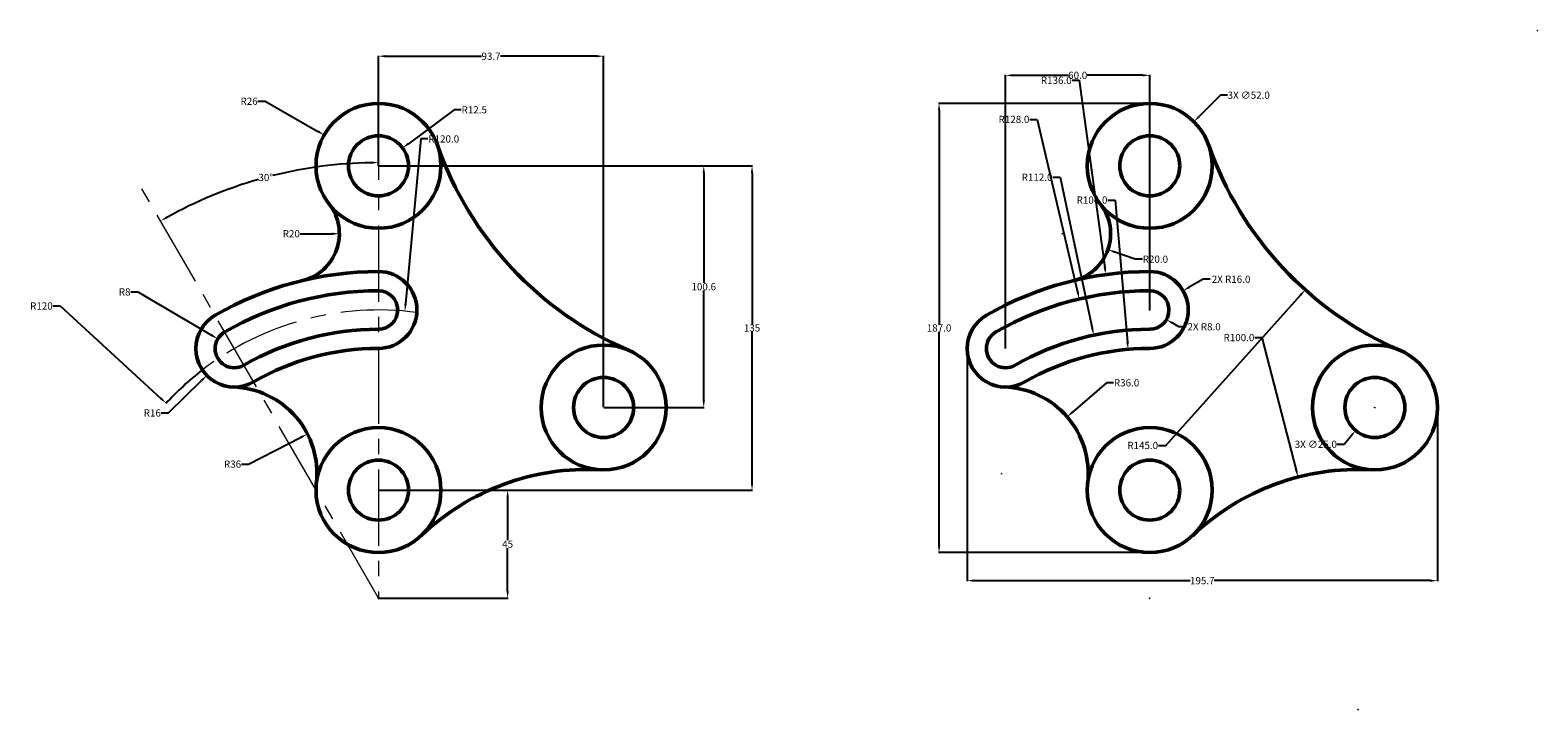
# Model space of a CAD drawing. Units: millimetres. Extents: x -10 to 618, y 0 to 283.
import ezdxf

# ---------------------------------------------------------------- set-up
doc = ezdxf.new("R2010")
doc.units = ezdxf.units.MM
doc.header["$MEASUREMENT"] = 0
doc.linetypes.add('CENTER', pattern=[50.8, 31.75, -6.35, 6.35, -6.35])
for name, color, linetype, lineweight in [('M-CNTR', 7, 'CENTER', 18), ('M-DIMS', 3, 'Continuous', 25), ('M-OUTL', 7, 'Continuous', 50)]:
    doc.layers.add(name, color=color, linetype=linetype, lineweight=lineweight)
doc.styles.get("Standard").update_dxf_attribs({"font": 'arial.ttf'})
doc.dimstyles.get("Standard").update_dxf_attribs({"dimtxt": 3, "dimasz": 3, "dimexe": 0.18, "dimexo": 0.0625, "dimgap": 0.09, "dimtad": 0, "dimtih": 1, "dimtoh": 1, "dimdec": 1, "dimdsep": 46, "dimtxsty": 'Standard', "dimcen": 0.09, "dimadec": 0, "dimazin": 0, "dimtfac": 1, "dimtdec": 1, "dimtofl": 0, "dimtmove": 0, "dimatfit": 3, "dimfxl": 1, "dimtolj": 1, "dimtzin": 0, "dimarcsym": 0})

# ---------------------------------------------------------------- blocks, each defined once
blk = doc.blocks.new('*D1')
at = {"layer": 'Defpoints', "color": 0, "transparency": 16777216}
for p in [(135.32, 252.15), (103.83, 224.75), (35.32, 219.36), (135.32, 46.15), (135.32, 46.15)]:
    blk.add_point(p, dxfattribs=at)
at = {"layer": 'M-DIMS', "color": 0, "lineweight": -2, "transparency": 16777216}
for start, end in [(90.94784, 104.01062), (105.99398, 119.05216)]:
    blk.add_arc((135.32, 46.15), 181.35, start, end, dxfattribs=at)
at = {"layer": 'M-DIMS', "color": 0, "transparency": 16777216}
for points in [[(132.32, 227.98), (132.33, 226.98), (135.32, 227.5)], [(47.51, 204.25), (47.01, 205.12), (44.65, 203.21)]]:
    blk.add_solid(points, dxfattribs=at)
at = {"layer": 'M-DIMS', "color": 0, "transparency": 16777216, "insert": (88.39, 221.32), "char_height": 3, "attachment_point": 5}
blk.add_mtext('\\A1;30°', dxfattribs=at)
blk = doc.blocks.new('*D2')
at = {"layer": 'Defpoints', "color": 0, "transparency": 16777216}
for p in [(99.04, 197.88), (119.04, 197.88)]:
    blk.add_point(p, dxfattribs=at)
at = {"layer": 'M-DIMS', "color": 0, "lineweight": -2, "transparency": 16777216}
blk.add_line((102.71, 197.88), (116.04, 197.88), dxfattribs=at)
at = {"layer": 'M-DIMS', "color": 0, "transparency": 16777216}
blk.add_solid([(116.04, 198.38), (116.04, 197.38), (119.04, 197.88)], dxfattribs=at)
at = {"layer": 'M-DIMS', "color": 0, "transparency": 16777216, "insert": (99.04, 197.88), "char_height": 3, "attachment_point": 5}
blk.add_mtext('\\A1;R20', dxfattribs=at)
blk = doc.blocks.new('*D3')
at = {"layer": 'Defpoints', "color": 0, "transparency": 16777216}
for p in [(135.32, 91.15), (189.08, 91.15), (135.32, 46.15)]:
    blk.add_point(p, dxfattribs=at)
at = {"layer": 'M-DIMS', "color": 0, "lineweight": -2, "transparency": 16777216}
for p, q in [((135.39, 91.15), (189.26, 91.15)), ((189.08, 88.15), (189.08, 70.27)), ((189.08, 49.15), (189.08, 67.04)), ((135.39, 46.15), (189.26, 46.15))]:
    blk.add_line(p, q, dxfattribs=at)
at = {"layer": 'M-DIMS', "color": 0, "transparency": 16777216}
for points in [[(188.58, 88.15), (189.58, 88.15), (189.08, 91.15)], [(188.58, 49.15), (189.58, 49.15), (189.08, 46.15)]]:
    blk.add_solid(points, dxfattribs=at)
at = {"layer": 'M-DIMS', "color": 0, "transparency": 16777216, "insert": (189.08, 68.65), "char_height": 3, "attachment_point": 5}
blk.add_mtext('\\A1;45', dxfattribs=at)
blk = doc.blocks.new('*D4')
at = {"layer": 'Defpoints', "color": 0, "transparency": 16777216}
for p in [(135.32, 226.15), (290.79, 226.15), (135.32, 91.15)]:
    blk.add_point(p, dxfattribs=at)
at = {"layer": 'M-DIMS', "color": 0, "lineweight": -2, "transparency": 16777216}
for p, q in [((135.39, 226.15), (290.97, 226.15)), ((290.79, 223.15), (290.79, 160.28)), ((290.79, 94.15), (290.79, 157.03)), ((135.39, 91.15), (290.97, 91.15))]:
    blk.add_line(p, q, dxfattribs=at)
at = {"layer": 'M-DIMS', "color": 0, "transparency": 16777216}
for points in [[(290.29, 223.15), (291.29, 223.15), (290.79, 226.15)], [(290.29, 94.15), (291.29, 94.15), (290.79, 91.15)]]:
    blk.add_solid(points, dxfattribs=at)
at = {"layer": 'M-DIMS', "color": 0, "transparency": 16777216, "insert": (290.79, 158.65), "char_height": 3, "attachment_point": 5}
blk.add_mtext('\\A1;135', dxfattribs=at)
blk = doc.blocks.new('*D5')
at = {"layer": 'Defpoints', "color": 0, "transparency": 16777216}
for p in [(135.32, 271.81), (135.32, 226.15), (229.02, 125.55)]:
    blk.add_point(p, dxfattribs=at)
at = {"layer": 'M-DIMS', "color": 0, "lineweight": -2, "transparency": 16777216}
for p, q in [((135.32, 226.22), (135.32, 271.99)), ((138.32, 271.81), (178.19, 271.81)), ((226.02, 271.81), (186.16, 271.81)), ((229.02, 125.62), (229.02, 271.99))]:
    blk.add_line(p, q, dxfattribs=at)
at = {"layer": 'M-DIMS', "color": 0, "transparency": 16777216}
for points in [[(138.32, 272.31), (138.32, 271.31), (135.32, 271.81)], [(226.02, 272.31), (226.02, 271.31), (229.02, 271.81)]]:
    blk.add_solid(points, dxfattribs=at)
at = {"layer": 'M-DIMS', "color": 0, "transparency": 16777216, "insert": (182.17, 271.81), "char_height": 3, "attachment_point": 5}
blk.add_mtext('\\A1;93.7', dxfattribs=at)
blk = doc.blocks.new('*D6')
at = {"layer": 'Defpoints', "color": 0, "transparency": 16777216}
for p in [(135.32, 226.15), (270.7, 226.15), (229.02, 125.55)]:
    blk.add_point(p, dxfattribs=at)
at = {"layer": 'M-DIMS', "color": 0, "lineweight": -2, "transparency": 16777216}
for p, q in [((135.39, 226.15), (270.88, 226.15)), ((270.7, 223.15), (270.7, 177.47)), ((270.7, 128.55), (270.7, 174.23)), ((229.09, 125.55), (270.88, 125.55))]:
    blk.add_line(p, q, dxfattribs=at)
at = {"layer": 'M-DIMS', "color": 0, "transparency": 16777216}
for points in [[(270.2, 223.15), (271.2, 223.15), (270.7, 226.15)], [(270.2, 128.55), (271.2, 128.55), (270.7, 125.55)]]:
    blk.add_solid(points, dxfattribs=at)
at = {"layer": 'M-DIMS', "color": 0, "transparency": 16777216, "insert": (270.7, 175.85), "char_height": 3, "attachment_point": 5}
blk.add_mtext('\\A1;100.6', dxfattribs=at)
blk = doc.blocks.new('*D7')
at = {"layer": 'Defpoints', "color": 0, "transparency": 16777216}
for p in [(75.32, 150.08), (63.87, 138.9)]:
    blk.add_point(p, dxfattribs=at)
at = {"layer": 'M-DIMS', "color": 0, "lineweight": -2, "transparency": 16777216}
for p, q in [((75.23, 150.08), (75.41, 150.08)), ((75.32, 149.99), (75.32, 150.17)), ((47.87, 123.28), (61.73, 136.8)), ((44.87, 123.28), (47.87, 123.28))]:
    blk.add_line(p, q, dxfattribs=at)
at = {"layer": 'M-DIMS', "color": 0, "transparency": 16777216}
blk.add_solid([(61.38, 137.16), (62.08, 136.45), (63.87, 138.9)], dxfattribs=at)
at = {"layer": 'M-DIMS', "color": 0, "transparency": 16777216, "insert": (41.2, 123.28), "char_height": 3, "attachment_point": 5}
blk.add_mtext('\\A1;R16', dxfattribs=at)
blk = doc.blocks.new('*D8')
at = {"layer": 'Defpoints', "color": 0, "transparency": 16777216}
for p in [(105.75, 114.53), (73.71, 98.1)]:
    blk.add_point(p, dxfattribs=at)
at = {"layer": 'M-DIMS', "color": 0, "lineweight": -2, "transparency": 16777216}
for p, q in [((81.25, 101.97), (103.08, 113.16)), ((78.25, 101.97), (81.25, 101.97))]:
    blk.add_line(p, q, dxfattribs=at)
at = {"layer": 'M-DIMS', "color": 0, "transparency": 16777216}
blk.add_solid([(102.85, 113.61), (103.31, 112.72), (105.75, 114.53)], dxfattribs=at)
at = {"layer": 'M-DIMS', "color": 0, "transparency": 16777216, "insert": (74.58, 101.97), "char_height": 3, "attachment_point": 5}
blk.add_mtext('\\A1;R36', dxfattribs=at)
blk = doc.blocks.new('*D9')
at = {"layer": 'Defpoints', "color": 0, "transparency": 16777216}
for p in [(46.95, 127.33), (135.32, 46.15)]:
    blk.add_point(p, dxfattribs=at)
at = {"layer": 'M-DIMS', "color": 0, "lineweight": -2, "transparency": 16777216}
for p, q in [((-0.11, 167.81), (2.89, 167.81)), ((2.89, 167.81), (44.74, 129.36)), ((135.23, 46.15), (135.41, 46.15)), ((135.32, 46.06), (135.32, 46.24))]:
    blk.add_line(p, q, dxfattribs=at)
blk.add_arc((135.32, 46.15), 120, 127.67495, 137.51567, dxfattribs=at)
at = {"layer": 'M-DIMS', "color": 0, "transparency": 16777216}
blk.add_solid([(45.08, 129.73), (44.4, 128.99), (46.95, 127.33)], dxfattribs=at)
at = {"layer": 'M-DIMS', "color": 0, "transparency": 16777216, "insert": (-4.95, 167.81), "char_height": 3, "attachment_point": 5}
blk.add_mtext('\\A1;R120', dxfattribs=at)
blk = doc.blocks.new('*D10')
at = {"layer": 'Defpoints', "color": 0, "transparency": 16777216}
for p in [(68.43, 154.13), (75.32, 150.08)]:
    blk.add_point(p, dxfattribs=at)
at = {"layer": 'M-DIMS', "color": 0, "lineweight": -2, "transparency": 16777216}
for p, q in [((32.2, 173.67), (35.2, 173.67)), ((35.2, 173.67), (65.84, 155.65)), ((75.23, 150.08), (75.41, 150.08)), ((75.32, 149.99), (75.32, 150.17))]:
    blk.add_line(p, q, dxfattribs=at)
at = {"layer": 'M-DIMS', "color": 0, "transparency": 16777216}
blk.add_solid([(66.1, 156.08), (65.59, 155.22), (68.43, 154.13)], dxfattribs=at)
at = {"layer": 'M-DIMS', "color": 0, "transparency": 16777216, "insert": (29.69, 173.67), "char_height": 3, "attachment_point": 5}
blk.add_mtext('\\A1;R8', dxfattribs=at)
blk = doc.blocks.new('*D11')
at = {"layer": 'Defpoints', "color": 0, "transparency": 16777216}
for p in [(112.74, 239.03), (135.32, 226.15)]:
    blk.add_point(p, dxfattribs=at)
at = {"layer": 'M-DIMS', "color": 0, "lineweight": -2, "transparency": 16777216}
for p, q in [((85.14, 253.05), (88.14, 253.05)), ((88.14, 253.05), (110.13, 240.52)), ((135.23, 226.15), (135.41, 226.15)), ((135.32, 226.06), (135.32, 226.24))]:
    blk.add_line(p, q, dxfattribs=at)
at = {"layer": 'M-DIMS', "color": 0, "transparency": 16777216}
blk.add_solid([(110.38, 240.95), (109.88, 240.08), (112.74, 239.03)], dxfattribs=at)
at = {"layer": 'M-DIMS', "color": 0, "transparency": 16777216, "insert": (81.47, 253.05), "char_height": 3, "attachment_point": 5}
blk.add_mtext('\\A1;R26', dxfattribs=at)
blk = doc.blocks.new('*D12')
at = {"layer": 'Defpoints', "color": 0, "transparency": 16777216}
for p in [(145.36, 233.6), (135.32, 226.15)]:
    blk.add_point(p, dxfattribs=at)
at = {"layer": 'M-DIMS', "color": 0, "lineweight": -2, "transparency": 16777216}
for p, q in [((166.76, 249.49), (147.77, 235.39)), ((169.76, 249.49), (166.76, 249.49)), ((135.23, 226.15), (135.41, 226.15)), ((135.32, 226.06), (135.32, 226.24))]:
    blk.add_line(p, q, dxfattribs=at)
at = {"layer": 'M-DIMS', "color": 0, "transparency": 16777216}
blk.add_solid([(147.47, 235.79), (148.07, 234.99), (145.36, 233.6)], dxfattribs=at)
at = {"layer": 'M-DIMS', "color": 0, "transparency": 16777216, "insert": (175.19, 249.49), "char_height": 3, "attachment_point": 5}
blk.add_mtext('\\A1;R12.5', dxfattribs=at)
blk = doc.blocks.new('LINKAGE-BRACKET-ARC-SLOT')
for centre, radius in [((76, 161), 26), ((76, 161), 12.5), ((169.7, 60.4), 26), ((169.7, 60.4), 12.5), ((76, 26), 26), ((76, 26), 12.5)]:
    blk.add_circle(centre, radius)
for centre, radius, start, end in [((237.43, 217.42), 145, 199.26409, 246.66823), ((39.72, 132.72), 20, 283.44875, 37.93262), ((76, -19), 136, 90, 120), ((76, 101), 16, 270, 90), ((76, -19), 128, 90, 120), ((76, 101), 8, 270, 90), ((16, 84.92), 16, 120, 300), ((16, 84.92), 8, 120, 300), ((76, -19), 112, 90, 120), ((76, -19), 104, 90, 120), ((14.39, 32.95), 36, 353.5657, 88.22634), ((162.72, -65.41), 100, 86.82559, 133.49373)]:
    blk.add_arc(centre, radius, start, end)
blk = doc.blocks.new('*D14')
at = {"layer": 'Defpoints', "color": 0, "transparency": 16777216}
for p in [(380.33, 150.08), (576.03, 125.55), (576.03, 53.45)]:
    blk.add_point(p, dxfattribs=at)
at = {"layer": 'M-DIMS', "color": 0, "lineweight": -2, "transparency": 16777216}
for p, q in [((380.33, 150.01), (380.33, 53.27)), ((576.03, 125.49), (576.03, 53.27)), ((383.33, 53.45), (473.17, 53.45)), ((573.03, 53.45), (483.19, 53.45))]:
    blk.add_line(p, q, dxfattribs=at)
at = {"layer": 'M-DIMS', "color": 0, "transparency": 16777216}
for points in [[(383.33, 53.95), (383.33, 52.95), (380.33, 53.45)], [(573.03, 53.95), (573.03, 52.95), (576.03, 53.45)]]:
    blk.add_solid(points, dxfattribs=at)
at = {"layer": 'M-DIMS', "color": 0, "transparency": 16777216, "insert": (478.18, 53.45), "char_height": 3, "attachment_point": 5}
blk.add_mtext('\\A1;195.7', dxfattribs=at)
blk = doc.blocks.new('*D15')
at = {"layer": 'Defpoints', "color": 0, "transparency": 16777216}
for p in [(368.63, 252.15), (456.33, 252.15), (456.33, 65.15)]:
    blk.add_point(p, dxfattribs=at)
at = {"layer": 'M-DIMS', "color": 0, "lineweight": -2, "transparency": 16777216}
for p, q in [((456.27, 252.15), (368.45, 252.15)), ((368.63, 249.15), (368.63, 160.27)), ((368.63, 68.15), (368.63, 157.03)), ((456.27, 65.15), (368.45, 65.15))]:
    blk.add_line(p, q, dxfattribs=at)
at = {"layer": 'M-DIMS', "color": 0, "transparency": 16777216}
for points in [[(368.13, 249.15), (369.13, 249.15), (368.63, 252.15)], [(368.13, 68.15), (369.13, 68.15), (368.63, 65.15)]]:
    blk.add_solid(points, dxfattribs=at)
at = {"layer": 'M-DIMS', "color": 0, "transparency": 16777216, "insert": (368.63, 158.65), "char_height": 3, "attachment_point": 5}
blk.add_mtext('\\A1;187.0', dxfattribs=at)
blk = doc.blocks.new('*D16')
at = {"layer": 'Defpoints', "color": 0, "transparency": 16777216}
for p in [(456.33, 263.85), (456.33, 166.15), (396.33, 150.08)]:
    blk.add_point(p, dxfattribs=at)
at = {"layer": 'M-DIMS', "color": 0, "lineweight": -2, "transparency": 16777216}
for p, q in [((396.33, 150.14), (396.33, 264.03)), ((399.33, 263.85), (422.34, 263.85)), ((453.33, 263.85), (430.32, 263.85)), ((456.33, 166.22), (456.33, 264.03))]:
    blk.add_line(p, q, dxfattribs=at)
at = {"layer": 'M-DIMS', "color": 0, "transparency": 16777216}
for points in [[(399.33, 264.35), (399.33, 263.35), (396.33, 263.85)], [(453.33, 264.35), (453.33, 263.35), (456.33, 263.85)]]:
    blk.add_solid(points, dxfattribs=at)
at = {"layer": 'M-DIMS', "color": 0, "transparency": 16777216, "insert": (426.33, 263.85), "char_height": 3, "attachment_point": 5}
blk.add_mtext('\\A1;60.0', dxfattribs=at)
blk = doc.blocks.new('*D17')
at = {"layer": 'Defpoints', "color": 0, "transparency": 16777216}
for p in [(146.32, 165.65), (135.32, 46.15)]:
    blk.add_point(p, dxfattribs=at)
at = {"layer": 'M-DIMS', "color": 0, "lineweight": -2, "transparency": 16777216}
for p, q in [((152.92, 237.35), (146.59, 168.64)), ((155.92, 237.35), (152.92, 237.35)), ((135.23, 46.15), (135.41, 46.15)), ((135.32, 46.06), (135.32, 46.24))]:
    blk.add_line(p, q, dxfattribs=at)
at = {"layer": 'M-DIMS', "color": 0, "transparency": 16777216}
blk.add_solid([(146.1, 168.68), (147.09, 168.59), (146.32, 165.65)], dxfattribs=at)
at = {"layer": 'M-DIMS', "color": 0, "transparency": 16777216, "insert": (162.5, 237.35), "char_height": 3, "attachment_point": 5}
blk.add_mtext('\\A1;R120.0', dxfattribs=at)
blk = doc.blocks.new('*D18')
at = {"layer": 'Defpoints', "color": 0, "transparency": 16777216}
for p in [(474.72, 244.54), (437.95, 207.77)]:
    blk.add_point(p, dxfattribs=at)
at = {"layer": 'M-DIMS', "color": 0, "lineweight": -2, "transparency": 16777216}
for p, q in [((485.75, 255.57), (476.84, 246.66)), ((488.75, 255.57), (485.75, 255.57)), ((456.24, 226.15), (456.42, 226.15)), ((456.33, 226.06), (456.33, 226.24))]:
    blk.add_line(p, q, dxfattribs=at)
at = {"layer": 'M-DIMS', "color": 0, "transparency": 16777216}
blk.add_solid([(476.48, 247.01), (477.19, 246.31), (474.72, 244.54)], dxfattribs=at)
at = {"layer": 'M-DIMS', "color": 0, "transparency": 16777216, "insert": (497.5, 255.57), "char_height": 3, "attachment_point": 5}
blk.add_mtext('\\A1;3X ∅52.0', dxfattribs=at)
blk = doc.blocks.new('*D19')
at = {"layer": 'Defpoints', "color": 0, "transparency": 16777216}
for p in [(558.06, 135.13), (542, 115.97)]:
    blk.add_point(p, dxfattribs=at)
at = {"layer": 'M-DIMS', "color": 0, "lineweight": -2, "transparency": 16777216}
for p, q in [((549.94, 125.55), (550.12, 125.55)), ((550.03, 125.46), (550.03, 125.64)), ((537.18, 110.22), (540.08, 113.67)), ((534.18, 110.22), (537.18, 110.22))]:
    blk.add_line(p, q, dxfattribs=at)
at = {"layer": 'M-DIMS', "color": 0, "transparency": 16777216}
blk.add_solid([(539.69, 113.99), (540.46, 113.35), (542, 115.97)], dxfattribs=at)
at = {"layer": 'M-DIMS', "color": 0, "transparency": 16777216, "insert": (525.43, 110.22), "char_height": 3, "attachment_point": 5}
blk.add_mtext('\\A1;3X ∅25.0', dxfattribs=at)
blk = doc.blocks.new('*D20')
at = {"layer": 'Defpoints', "color": 0, "transparency": 16777216}
for p in [(420.05, 197.88), (438.92, 191.26)]:
    blk.add_point(p, dxfattribs=at)
at = {"layer": 'M-DIMS', "color": 0, "lineweight": -2, "transparency": 16777216}
for p, q in [((419.96, 197.88), (420.14, 197.88)), ((420.05, 197.79), (420.05, 197.97)), ((450.25, 187.29), (441.76, 190.27)), ((453.25, 187.29), (450.25, 187.29))]:
    blk.add_line(p, q, dxfattribs=at)
at = {"layer": 'M-DIMS', "color": 0, "transparency": 16777216}
blk.add_solid([(441.92, 190.74), (441.59, 189.8), (438.92, 191.26)], dxfattribs=at)
at = {"layer": 'M-DIMS', "color": 0, "transparency": 16777216, "insert": (458.67, 187.29), "char_height": 3, "attachment_point": 5}
blk.add_mtext('\\A1;R20.0', dxfattribs=at)
blk = doc.blocks.new('*D21')
at = {"layer": 'Defpoints', "color": 0, "transparency": 16777216}
for p in [(421.93, 121.67), (394.72, 98.1)]:
    blk.add_point(p, dxfattribs=at)
at = {"layer": 'M-DIMS', "color": 0, "lineweight": -2, "transparency": 16777216}
for p, q in [((438.26, 135.81), (424.2, 123.63)), ((441.26, 135.81), (438.26, 135.81)), ((394.63, 98.1), (394.81, 98.1)), ((394.72, 98.01), (394.72, 98.19))]:
    blk.add_line(p, q, dxfattribs=at)
at = {"layer": 'M-DIMS', "color": 0, "transparency": 16777216}
blk.add_solid([(423.87, 124.01), (424.53, 123.26), (421.93, 121.67)], dxfattribs=at)
at = {"layer": 'M-DIMS', "color": 0, "transparency": 16777216, "insert": (446.68, 135.81), "char_height": 3, "attachment_point": 5}
blk.add_mtext('\\A1;R36.0', dxfattribs=at)
blk = doc.blocks.new('*D22')
at = {"layer": 'Defpoints', "color": 0, "transparency": 16777216}
for p in [(617.76, 282.57), (521.02, 174.56)]:
    blk.add_point(p, dxfattribs=at)
at = {"layer": 'M-DIMS', "color": 0, "lineweight": -2, "transparency": 16777216}
for p, q in [((617.67, 282.57), (617.85, 282.57)), ((617.76, 282.48), (617.76, 282.66)), ((462.97, 109.75), (519.01, 172.32)), ((459.97, 109.75), (462.97, 109.75))]:
    blk.add_line(p, q, dxfattribs=at)
at = {"layer": 'M-DIMS', "color": 0, "transparency": 16777216}
blk.add_solid([(518.64, 172.66), (519.39, 171.99), (521.02, 174.56)], dxfattribs=at)
at = {"layer": 'M-DIMS', "color": 0, "transparency": 16777216, "insert": (453.39, 109.75), "char_height": 3, "attachment_point": 5}
blk.add_mtext('\\A1;R145.0', dxfattribs=at)
blk = doc.blocks.new('*D23')
at = {"layer": 'Defpoints', "color": 0, "transparency": 16777216}
for p in [(518.04, 96.57), (543.05, -0.25)]:
    blk.add_point(p, dxfattribs=at)
at = {"layer": 'M-DIMS', "color": 0, "lineweight": -2, "transparency": 16777216}
for p, q in [((500.03, 154.66), (503.03, 154.66)), ((503.03, 154.66), (517.29, 99.47)), ((542.96, -0.25), (543.14, -0.25)), ((543.05, -0.34), (543.05, -0.16))]:
    blk.add_line(p, q, dxfattribs=at)
at = {"layer": 'M-DIMS', "color": 0, "transparency": 16777216}
blk.add_solid([(517.77, 99.6), (516.81, 99.35), (518.04, 96.57)], dxfattribs=at)
at = {"layer": 'M-DIMS', "color": 0, "transparency": 16777216, "insert": (493.45, 154.66), "char_height": 3, "attachment_point": 5}
blk.add_mtext('\\A1;R100.0', dxfattribs=at)
blk = doc.blocks.new('*D24')
at = {"layer": 'Defpoints', "color": 0, "transparency": 16777216}
for p in [(470.19, 174.15), (456.33, 166.15)]:
    blk.add_point(p, dxfattribs=at)
at = {"layer": 'M-DIMS', "color": 0, "lineweight": -2, "transparency": 16777216}
for p, q in [((478.5, 178.95), (472.79, 175.65)), ((481.5, 178.95), (478.5, 178.95)), ((456.24, 166.15), (456.42, 166.15)), ((456.33, 166.06), (456.33, 166.24))]:
    blk.add_line(p, q, dxfattribs=at)
at = {"layer": 'M-DIMS', "color": 0, "transparency": 16777216}
blk.add_solid([(472.54, 176.09), (473.04, 175.22), (470.19, 174.15)], dxfattribs=at)
at = {"layer": 'M-DIMS', "color": 0, "transparency": 16777216, "insert": (490.17, 178.95), "char_height": 3, "attachment_point": 5}
blk.add_mtext('\\A1;2X R16.0', dxfattribs=at)
blk = doc.blocks.new('*D25')
at = {"layer": 'Defpoints', "color": 0, "transparency": 16777216}
for p in [(456.33, 166.15), (463.26, 162.15)]:
    blk.add_point(p, dxfattribs=at)
at = {"layer": 'M-DIMS', "color": 0, "lineweight": -2, "transparency": 16777216}
for p, q in [((456.24, 166.15), (456.42, 166.15)), ((456.33, 166.06), (456.33, 166.24)), ((468.45, 159.15), (465.86, 160.65)), ((471.45, 159.15), (468.45, 159.15))]:
    blk.add_line(p, q, dxfattribs=at)
at = {"layer": 'M-DIMS', "color": 0, "transparency": 16777216}
blk.add_solid([(466.11, 161.08), (465.61, 160.22), (463.26, 162.15)], dxfattribs=at)
at = {"layer": 'M-DIMS', "color": 0, "transparency": 16777216, "insert": (478.95, 159.15), "char_height": 3, "attachment_point": 5}
blk.add_mtext('\\A1;2X R8.0', dxfattribs=at)
blk = doc.blocks.new('*D26')
at = {"layer": 'Defpoints', "color": 0, "transparency": 16777216}
for p in [(438, 180.91), (456.33, 46.15)]:
    blk.add_point(p, dxfattribs=at)
at = {"layer": 'M-DIMS', "color": 0, "lineweight": -2, "transparency": 16777216}
for p, q in [((424, 261.77), (427, 261.77)), ((427, 261.77), (437.6, 183.88)), ((456.24, 46.15), (456.42, 46.15)), ((456.33, 46.06), (456.33, 46.24))]:
    blk.add_line(p, q, dxfattribs=at)
at = {"layer": 'M-DIMS', "color": 0, "transparency": 16777216}
blk.add_solid([(438.09, 183.95), (437.1, 183.82), (438, 180.91)], dxfattribs=at)
at = {"layer": 'M-DIMS', "color": 0, "transparency": 16777216, "insert": (417.42, 261.77), "char_height": 3, "attachment_point": 5}
blk.add_mtext('\\A1;R136.0', dxfattribs=at)
blk = doc.blocks.new('*D27')
at = {"layer": 'Defpoints', "color": 0, "transparency": 16777216}
for p in [(427, 170.75), (456.33, 46.15)]:
    blk.add_point(p, dxfattribs=at)
at = {"layer": 'M-DIMS', "color": 0, "lineweight": -2, "transparency": 16777216}
for p, q in [((406.4, 245.5), (409.4, 245.5)), ((409.4, 245.5), (426.31, 173.67)), ((456.24, 46.15), (456.42, 46.15)), ((456.33, 46.06), (456.33, 46.24))]:
    blk.add_line(p, q, dxfattribs=at)
at = {"layer": 'M-DIMS', "color": 0, "transparency": 16777216}
blk.add_solid([(426.8, 173.78), (425.82, 173.55), (427, 170.75)], dxfattribs=at)
at = {"layer": 'M-DIMS', "color": 0, "transparency": 16777216, "insert": (399.82, 245.5), "char_height": 3, "attachment_point": 5}
blk.add_mtext('\\A1;R128.0', dxfattribs=at)
blk = doc.blocks.new('*D28')
at = {"layer": 'Defpoints', "color": 0, "transparency": 16777216}
for p in [(433, 155.7), (456.33, 46.15)]:
    blk.add_point(p, dxfattribs=at)
at = {"layer": 'M-DIMS', "color": 0, "lineweight": -2, "transparency": 16777216}
for p, q in [((416, 221.42), (419, 221.42)), ((419, 221.42), (432.38, 158.63)), ((456.24, 46.15), (456.42, 46.15)), ((456.33, 46.06), (456.33, 46.24))]:
    blk.add_line(p, q, dxfattribs=at)
at = {"layer": 'M-DIMS', "color": 0, "transparency": 16777216}
blk.add_solid([(432.86, 158.73), (431.89, 158.53), (433, 155.7)], dxfattribs=at)
at = {"layer": 'M-DIMS', "color": 0, "transparency": 16777216, "insert": (409.42, 221.42), "char_height": 3, "attachment_point": 5}
blk.add_mtext('\\A1;R112.0', dxfattribs=at)
blk = doc.blocks.new('*D29')
at = {"layer": 'Defpoints', "color": 0, "transparency": 16777216}
for p in [(447.3, 149.76), (456.33, 46.15)]:
    blk.add_point(p, dxfattribs=at)
at = {"layer": 'M-DIMS', "color": 0, "lineweight": -2, "transparency": 16777216}
for p, q in [((438.88, 211.92), (441.88, 211.92)), ((441.88, 211.92), (447.04, 152.75)), ((456.24, 46.15), (456.42, 46.15)), ((456.33, 46.06), (456.33, 46.24))]:
    blk.add_line(p, q, dxfattribs=at)
at = {"layer": 'M-DIMS', "color": 0, "transparency": 16777216}
blk.add_solid([(447.54, 152.79), (446.54, 152.71), (447.3, 149.76)], dxfattribs=at)
at = {"layer": 'M-DIMS', "color": 0, "transparency": 16777216, "insert": (432.3, 211.92), "char_height": 3, "attachment_point": 5}
blk.add_mtext('\\A1;R104.0', dxfattribs=at)

msp = doc.modelspace()

# ---------------------------------------------------------------- linework, layer by layer
at = {"layer": 'M-CNTR'}
for p, q in [((135.32, 252.15), (135.32, 46.15)), ((135.32, 46.15), (35.32, 219.36))]:
    msp.add_line(p, q, dxfattribs=at)
msp.add_arc((135.32, 46.15), 120, 82.35489, 127.64511, dxfattribs=at)

# ---------------------------------------------------------------- block references
at = {"layer": 'M-OUTL'}
for p in [(59.32, 65.15), (380.33, 65.15)]:
    msp.add_blockref('LINKAGE-BRACKET-ARC-SLOT', p, dxfattribs=at)

# ---------------------------------------------------------------- dimensions: what is measured, and where the dimension line sits
at = {"layer": 'M-DIMS'}
for center, mpoint, picture, middle in [((617.76, 282.57), (521.02, 174.56), '*D22', (453.39, 109.75)), ((456.33, 46.15), (438, 180.91), '*D26', (417.42, 261.77)), ((456.33, 46.15), (427, 170.75), '*D27', (399.82, 245.5)), ((135.32, 46.15), (146.32, 165.65), '*D17', (162.5, 237.35)), ((456.33, 46.15), (433, 155.7), '*D28', (409.42, 221.42)), ((456.33, 46.15), (447.3, 149.76), '*D29', (432.3, 211.92)), ((420.05, 197.88), (438.92, 191.26), '*D20', (458.67, 187.29)), ((543.05, -0.25), (518.04, 96.57), '*D23', (493.45, 154.66)), ((394.72, 98.1), (421.93, 121.67), '*D21', (446.68, 135.81))]:
    dim = msp.add_radius_dim(center=center, mpoint=mpoint, dimstyle='Standard', override={"dimdec": 1, "dimlfac": 1, "dimrnd": 0, "dimzin": 0, "dimdsep": 46, "dimlunit": 2}, dxfattribs=at)
    dim.commit()
    dim.dimension.update_dxf_attribs({"geometry": picture, "text_midpoint": middle, "dimtype": 164})
at = {"layer": 'M-DIMS', "transparency": 33554610}
dim = msp.add_linear_dim(base=(135.32, 271.81), p1=(229.02, 125.55), p2=(135.32, 226.15), dimstyle='Standard', override={"dimclrd": 0, "dimclre": 0, "dimclrt": 0}, dxfattribs=at)
dim.commit()
dim.dimension.update_dxf_attribs({"geometry": '*D5', "text_midpoint": (182.17, 271.81)})
at = {"layer": 'M-DIMS'}
for base, p1, p2, picture, middle in [((456.33, 263.85), (396.33, 150.08), (456.33, 166.15), '*D16', (426.33, 263.85)), ((576.03, 53.45), (380.33, 150.08), (576.03, 125.55), '*D14', (478.18, 53.45))]:
    dim = msp.add_linear_dim(base=base, p1=p1, p2=p2, dimstyle='Standard', override={"dimdec": 1, "dimlfac": 1, "dimrnd": 0, "dimzin": 0, "dimdsep": 46, "dimlunit": 2}, dxfattribs=at)
    dim.commit()
    dim.dimension.update_dxf_attribs({"geometry": picture, "text_midpoint": middle})
for p1, p2, picture, middle in [((437.95, 207.77), (474.72, 244.54), '*D18', (497.5, 255.57)), ((558.06, 135.13), (542, 115.97), '*D19', (525.43, 110.22))]:
    dim = msp.add_diameter_dim_2p(p1=p1, p2=p2, text='3X <>', dimstyle='Standard', override={"dimdec": 1, "dimlfac": 1, "dimrnd": 0, "dimzin": 0, "dimdsep": 46, "dimlunit": 2}, dxfattribs=at)
    dim.commit()
    dim.dimension.update_dxf_attribs({"geometry": picture, "text_midpoint": middle, "dimtype": 163})
at = {"layer": 'M-DIMS', "transparency": 33554610}
dim = msp.add_angular_dim_2l(base=(103.83, 224.75), line1=((135.32, 252.15), (135.32, 46.15)), line2=((135.32, 46.15), (35.32, 219.36)), dimstyle='Standard', override={"dimclrd": 0, "dimclre": 0, "dimclrt": 0}, dxfattribs=at)
dim.commit()
dim.dimension.update_dxf_attribs({"geometry": '*D1', "text_midpoint": (88.39, 221.32)})
for center, mpoint, picture, middle in [((135.32, 226.15), (112.74, 239.03), '*D11', (81.47, 253.05)), ((135.32, 226.15), (145.36, 233.6), '*D12', (175.19, 249.49)), ((99.04, 197.88), (119.04, 197.88), '*D2', (99.04, 197.88)), ((135.32, 46.15), (46.95, 127.33), '*D9', (-4.95, 167.81)), ((75.32, 150.08), (68.43, 154.13), '*D10', (29.69, 173.67)), ((75.32, 150.08), (63.87, 138.9), '*D7', (41.2, 123.28)), ((73.71, 98.1), (105.75, 114.53), '*D8', (74.58, 101.97))]:
    dim = msp.add_radius_dim(center=center, mpoint=mpoint, dimstyle='Standard', override={"dimclrd": 0, "dimclre": 0, "dimclrt": 0}, dxfattribs=at)
    dim.commit()
    dim.dimension.update_dxf_attribs({"geometry": picture, "text_midpoint": middle, "dimtype": 164})
at = {"layer": 'M-DIMS'}
dim = msp.add_linear_dim(base=(368.63, 252.15), p1=(456.33, 65.15), p2=(456.33, 252.15), angle=90, dimstyle='Standard', override={"dimdec": 1, "dimlfac": 1, "dimrnd": 0, "dimzin": 0, "dimdsep": 46, "dimlunit": 2}, dxfattribs=at)
dim.commit()
dim.dimension.update_dxf_attribs({"geometry": '*D15', "text_midpoint": (368.63, 158.65)})
at = {"layer": 'M-DIMS', "transparency": 33554610}
dim = msp.add_aligned_dim(p1=(135.32, 91.15), p2=(135.32, 226.15), distance=-155.47, dimstyle='Standard', override={"dimclrd": 0, "dimclre": 0, "dimclrt": 0}, dxfattribs=at)
dim.commit()
dim.dimension.update_dxf_attribs({"geometry": '*D4', "text_midpoint": (290.79, 158.65)})
for base, p1, p2, picture, middle in [((270.7, 226.15), (229.02, 125.55), (135.32, 226.15), '*D6', (270.7, 175.85)), ((189.08, 91.15), (135.32, 46.15), (135.32, 91.15), '*D3', (189.08, 68.65))]:
    dim = msp.add_linear_dim(base=base, p1=p1, p2=p2, angle=90, dimstyle='Standard', override={"dimclrd": 0, "dimclre": 0, "dimclrt": 0}, dxfattribs=at)
    dim.commit()
    dim.dimension.update_dxf_attribs({"geometry": picture, "text_midpoint": middle})
at = {"layer": 'M-DIMS'}
dim = msp.add_radius_dim(center=(456.33, 166.15), mpoint=(470.19, 174.15), text='2X <>', dimstyle='Standard', override={"dimdec": 1, "dimlfac": 1, "dimrnd": 0, "dimzin": 0, "dimdsep": 46, "dimlunit": 2}, dxfattribs=at)
dim.commit()
dim.dimension.update_dxf_attribs({"geometry": '*D24', "text_midpoint": (490.17, 178.95), "dimtype": 164})
dim = msp.add_radius_dim(center=(456.33, 166.15), mpoint=(463.26, 162.15), text='2X <>', dimstyle='Standard', override={"dimdec": 1, "dimlfac": 1, "dimrnd": 0, "dimzin": 0, "dimdsep": 46, "dimlunit": 2}, dxfattribs=at)
dim.commit()
dim.dimension.update_dxf_attribs({"geometry": '*D25', "text_midpoint": (478.95, 159.15)})

doc.saveas('drawing.dxf')
